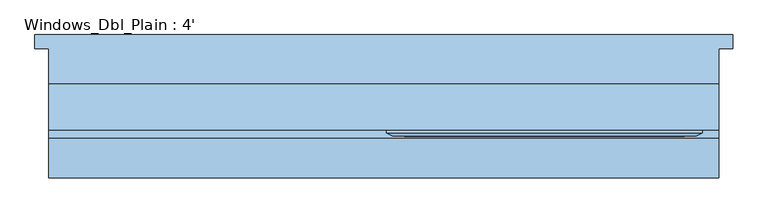
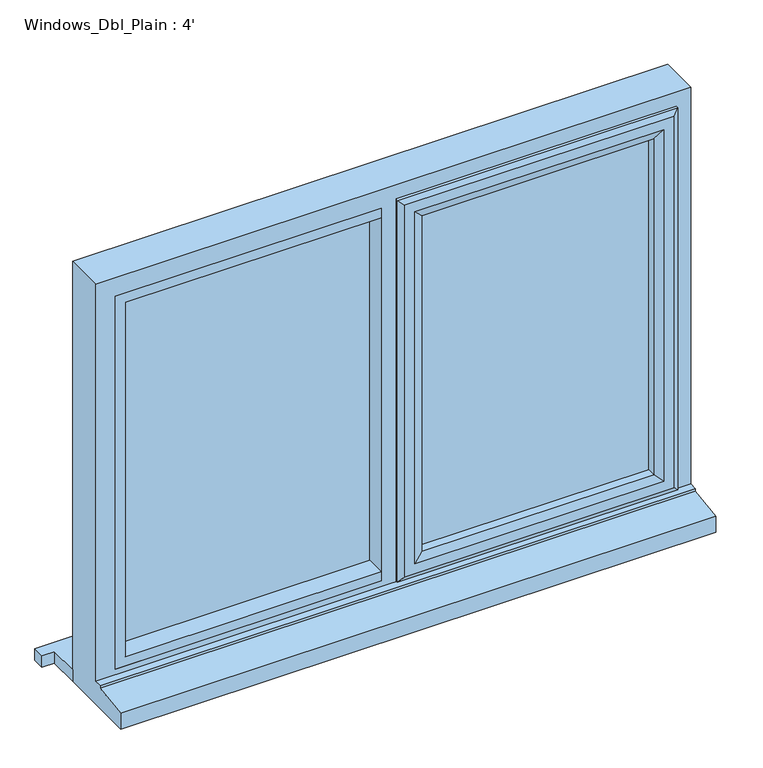
"""IFC4 building model written with IfcOpenShell, lengths in millimetres: window geometry, Windows_Dbl_Plain : 4'."""

from ifc_helpers import new_model, si_unit, frame, origin, place, context, project, spatial, polyline, outline, extrude, faceted_brep, source, transform, mapped, element, save


def windows_dbl_plain_4_4d10fa92(model_context):
    return source(origin(), model_context, "Body", "SolidModel", [
        extrude(outline(polyline([(-919.6, 115.6034322), (349.6, 115.6034322), (349.6, 90.6034322), (324.6, 90.6034322), (324.6, 25.4834322), (-894.6, 25.4834322), (-894.6, 90.6034322), (-919.6, 90.6034322), (-919.6, 115.6034322)])), frame((0.0, 0.0, 1200.0), z_axis=(0.0, 0.0, 1.0), x_axis=(1.0, 0.0, 0.0)), (0.0, 0.0, 1.0), 25.0),
        faceted_brep([(-280.0, -57.5165678, 2080.0), (-280.0, -57.5165678, 1253.0), (-280.0, -63.2900705, 1253.0), (-280.0, -63.2900705, 2080.0), (-270.0, 7.4834322, 2070.0), (-270.0, 7.4834322, 1263.0), (-270.0, -57.5165678, 1263.0), (-270.0, -57.5165678, 2070.0), (-230.0, -7.0094677, 2030.0), (-230.0, -7.0094677, 1303.0), (-240.1480377, 7.4834322, 1292.8519623), (-240.1480377, 7.4834322, 2040.1480377), (-230.0, -21.5165678, 2030.0), (-230.0, -21.5165678, 1303.0), (-240.0, -45.5165678, 2040.0), (-240.0, -45.5165678, 1293.0), (-240.0, -21.5165678, 1293.0), (-240.0, -21.5165678, 2040.0), (-230.0, -63.2900705, 2030.0), (-230.0, -63.2900705, 1303.0), (-230.0, -45.5165678, 1303.0), (-230.0, -45.5165678, 2030.0), (-247.4457548, -69.0635732, 2047.4457548), (-247.4457548, -69.0635732, 1285.5542452), (-269.2153903, -69.0635732, 1263.7846097), (-269.2153903, -69.0635732, 2069.2153903), (294.6, -57.5165678, 1253.0), (294.6, -63.2900705, 1253.0), (284.6, 7.4834322, 1263.0), (284.6, -57.5165678, 1263.0), (244.6, -7.0094677, 1303.0), (254.7480377, 7.4834322, 1292.8519623), (244.6, -21.5165678, 1303.0), (254.6, -45.5165678, 1293.0), (254.6, -21.5165678, 1293.0), (244.6, -63.2900705, 1303.0), (244.6, -45.5165678, 1303.0), (262.0457548, -69.0635732, 1285.5542452), (283.8153903, -69.0635732, 1263.7846097), (294.6, -57.5165678, 2080.0), (294.6, -63.2900705, 2080.0), (284.6, 7.4834322, 2070.0), (284.6, -57.5165678, 2070.0), (244.6, -7.0094677, 2030.0), (254.7480377, 7.4834322, 2040.1480377), (244.6, -21.5165678, 2030.0), (254.6, -45.5165678, 2040.0), (254.6, -21.5165678, 2040.0), (244.6, -63.2900705, 2030.0), (244.6, -45.5165678, 2030.0), (262.0457548, -69.0635732, 2047.4457548), (283.8153903, -69.0635732, 2069.2153903)], [[[0, 1, 2, 3]], [[4, 5, 6, 7]], [[8, 9, 10, 11]], [[12, 13, 9, 8]], [[14, 15, 16, 17]], [[18, 19, 20, 21]], [[22, 23, 19, 18]], [[3, 2, 24, 25]], [[1, 26, 27, 2]], [[5, 28, 29, 6]], [[9, 30, 31, 10]], [[13, 32, 30, 9]], [[15, 33, 34, 16]], [[19, 35, 36, 20]], [[23, 37, 35, 19]], [[2, 27, 38, 24]], [[26, 39, 40, 27]], [[28, 41, 42, 29]], [[30, 43, 44, 31]], [[32, 45, 43, 30]], [[33, 46, 47, 34]], [[35, 48, 49, 36]], [[37, 50, 48, 35]], [[27, 40, 51, 38]], [[39, 0, 3, 40]], [[1, 0, 39, 26], [7, 6, 29, 42]], [[41, 4, 7, 42]], [[5, 4, 41, 28], [11, 10, 31, 44]], [[43, 8, 11, 44]], [[45, 12, 8, 43]], [[17, 16, 34, 47], [13, 12, 45, 32]], [[46, 14, 17, 47]], [[15, 14, 46, 33], [21, 20, 36, 49]], [[48, 18, 21, 49]], [[50, 22, 18, 48]], [[25, 24, 38, 51], [23, 22, 50, 37]], [[40, 3, 25, 51]]]),
        extrude(outline(polyline([(2070.0, -310.0), (2070.0, -854.6), (1263.0, -854.6), (1263.0, -310.0), (1283.0, -310.0), (1283.0, -834.6), (2050.0, -834.6), (2050.0, -310.0), (2070.0, -310.0)])), frame((0.0, -57.5165678, 0.0), z_axis=(0.0, 1.0, 0.0), x_axis=(0.0, 0.0, 1.0)), (0.0, 0.0, 1.0), 41.0),
        faceted_brep([(324.6, 25.4834322, 2110.0), (324.6, 25.4834322, 1200.0), (-894.6, 25.4834322, 1200.0), (-894.6, 25.4834322, 2110.0), (264.6, 25.4834322, 2050.0), (-252.0, 25.4834322, 2050.0), (-252.0, 25.4834322, 1275.0), (264.6, 25.4834322, 1275.0), (-310.0, 25.4834322, 2050.0), (-834.6, 25.4834322, 2050.0), (-834.6, 25.4834322, 1275.0), (-310.0, 25.4834322, 1275.0), (-894.6, -145.0165678, 1200.0), (-894.6, -145.0165678, 1233.8088847), (-894.6, -72.5165678, 1244.7449676), (-894.6, -72.5165678, 1249.68767), (-894.6, -57.5165678, 1251.0), (-894.6, -57.5165678, 2110.0), (324.6, -57.5165678, 1251.0), (324.6, -57.5165678, 2110.0), (-854.6, -57.5165678, 2070.0), (-310.0, -57.5165678, 2070.0), (-310.0, -57.5165678, 1263.0), (-854.6, -57.5165678, 1263.0), (-270.0, -57.5165678, 2070.0), (284.6, -57.5165678, 2070.0), (284.6, -57.5165678, 1263.0), (-270.0, -57.5165678, 1263.0), (-854.6, 7.4834322, 1263.0), (-854.6, 7.4834322, 2070.0), (-300.0, 7.4834322, 1263.0), (-300.0, 7.4834322, 2070.0), (-310.0, 7.4834322, 2050.0), (-310.0, 7.4834322, 1275.0), (-834.6, 7.4834322, 1275.0), (-834.6, 7.4834322, 2050.0), (-270.0, 7.4834322, 2070.0), (-270.0, 7.4834322, 1263.0), (284.6, 7.4834322, 1263.0), (284.6, 7.4834322, 2070.0), (264.6, 7.4834322, 2050.0), (264.6, 7.4834322, 1275.0), (-252.0, 7.4834322, 1275.0), (-252.0, 7.4834322, 2050.0), (-300.0, -16.5165678, 2070.0), (-310.0, -16.5165678, 2070.0), (324.6, -72.5165678, 1249.68767), (324.6, -72.5165678, 1244.7449676), (324.6, -145.0165678, 1233.8088847), (324.6, -145.0165678, 1200.0), (-300.0, -16.5165678, 1263.0), (-310.0, -16.5165678, 1263.0)], [[[0, 1, 2, 3], [4, 5, 6, 7], [8, 9, 10, 11]], [[2, 12, 13, 14, 15, 16, 17, 3]], [[16, 18, 19, 17], [20, 21, 22, 23], [24, 25, 26, 27]], [[23, 28, 29, 20]], [[29, 28, 30, 31], [32, 33, 34, 35]], [[36, 37, 38, 39], [40, 41, 42, 43]], [[35, 34, 10, 9]], [[3, 17, 19, 0]], [[25, 24, 36, 39]], [[29, 31, 44, 45, 21, 20]], [[9, 8, 32, 35]], [[40, 43, 5, 4]], [[18, 46, 47, 48, 49, 1, 0, 19]], [[25, 39, 38, 26]], [[4, 7, 41, 40]], [[44, 31, 30, 50]], [[50, 51, 45, 44]], [[51, 22, 21, 45]], [[27, 37, 36, 24]], [[43, 42, 6, 5]], [[8, 11, 33, 32]], [[49, 12, 2, 1]], [[48, 13, 12, 49]], [[47, 14, 13, 48]], [[46, 15, 14, 47]], [[18, 16, 15, 46]], [[26, 38, 37, 27]], [[22, 51, 50, 30, 28, 23]], [[6, 42, 41, 7]], [[33, 11, 10, 34]]]),
        extrude(outline(polyline([(-854.6, -16.5165678), (-854.6, 7.4834322), (-300.0, 7.4834322), (-300.0, -16.5165678), (-854.6, -16.5165678)])), frame((0.0, 0.0, 1263.0), z_axis=(0.0, 0.0, 1.0), x_axis=(1.0, 0.0, 0.0)), (0.0, 0.0, 1.0), 807.0),
        extrude(outline(polyline([(254.6, -21.5165678), (254.6, -45.5165678), (-240.0, -45.5165678), (-240.0, -21.5165678), (254.6, -21.5165678)])), frame((0.0, 0.0, 1293.0), z_axis=(0.0, 0.0, 1.0), x_axis=(1.0, 0.0, 0.0)), (0.0, 0.0, 1.0), 747.0),
    ])


if __name__ == "__main__":
    model = new_model("IFC4")
    model_context = context("Model", 3, world=origin())
    ifc_project = project(units=[si_unit("LENGTHUNIT", "METRE", prefix="MILLI")], contexts=[model_context])
    site = spatial("IfcSite", under=ifc_project)
    building = spatial("IfcBuilding", under=site)
    placement = place(None, origin())
    windows_dbl_plain_4_shape = windows_dbl_plain_4_4d10fa92(model_context)
    element("IfcWindow", 1, ObjectType="Windows_Dbl_Plain : 4'", at=placement, inside=building, context=model_context, shape_type="MappedRepresentation", body=[
        mapped(windows_dbl_plain_4_shape, transform((0.0, 0.0, 0.0), x_axis=(1.0, 0.0, 0.0), y_axis=(0.0, 1.0, 0.0), z_axis=(0.0, 0.0, 1.0))),
    ])
    save(model, "model.ifc")

# Revit data of these elements
# Type "Windows_Dbl_Plain : 4'"
#   Type Mark = "56"
#   Operation = "DoublePanelVertical"
#   Construction Type Id = "GSP4R"
#   Manufacturer = "Revit"
#   Keynote = "L10"
#   Analytic Construction = "1/8 in Pilkington single glazing"
#   Wrap Layers (Ext) from Ext = 0.336286 ft
#   Wrap Layers (Int) from Ext = 0.582349 ft
#   Window Board Projection = 0.082021 ft
#   Window Board Extension = 0.082021 ft
#   Visual Light Transmittance = 0.9
#   Solar Heat Gain Coefficient = 0.78
#   Rough Width = 4.0 ft
#   Rough Height = 2.985564 ft
#   Height = 2.985564 ft
#   Width = 4.0 ft
#   Heat Transfer Coefficient (U) = 3.6886 W/(m²·K)
#   Glazing Thickness = 0.07874 ft
#   FrameOffset - External = 0.164042 ft
#   Frame Depth = 0.213255 ft
#   Default Head Height = 6.922572 ft
#   Cill Depth = 0.287073 ft
#   Cavity Closer Width = 0.164042 ft
#   Cavity Closer Offset from Ext = 0.336286 ft
#   Cavity Closer Depth = 0.278871 ft
#   Vis - Cavity Closers = yes
#   Define Thermal Properties by = 1
#   Material Trim = Window Frame
#   Material Glass = Glass
#   Material Frame = Window Frame
#   Wall Closure = (empty or 0)
# Element 1 (IfcWindow, "Windows_Dbl_Plain : 4'")
#   Materials on its faces: "Window Frame", "Glass"
# Materials
#   "Window Frame": colour RGB 249 249 249, transparency 0, Keynote = "L10", Cost = 0
#   "Glass": class "Glass", colour RGB 0 128 192, transparency 0.9, Description = "Soda Lime Glass", Cost = 0
